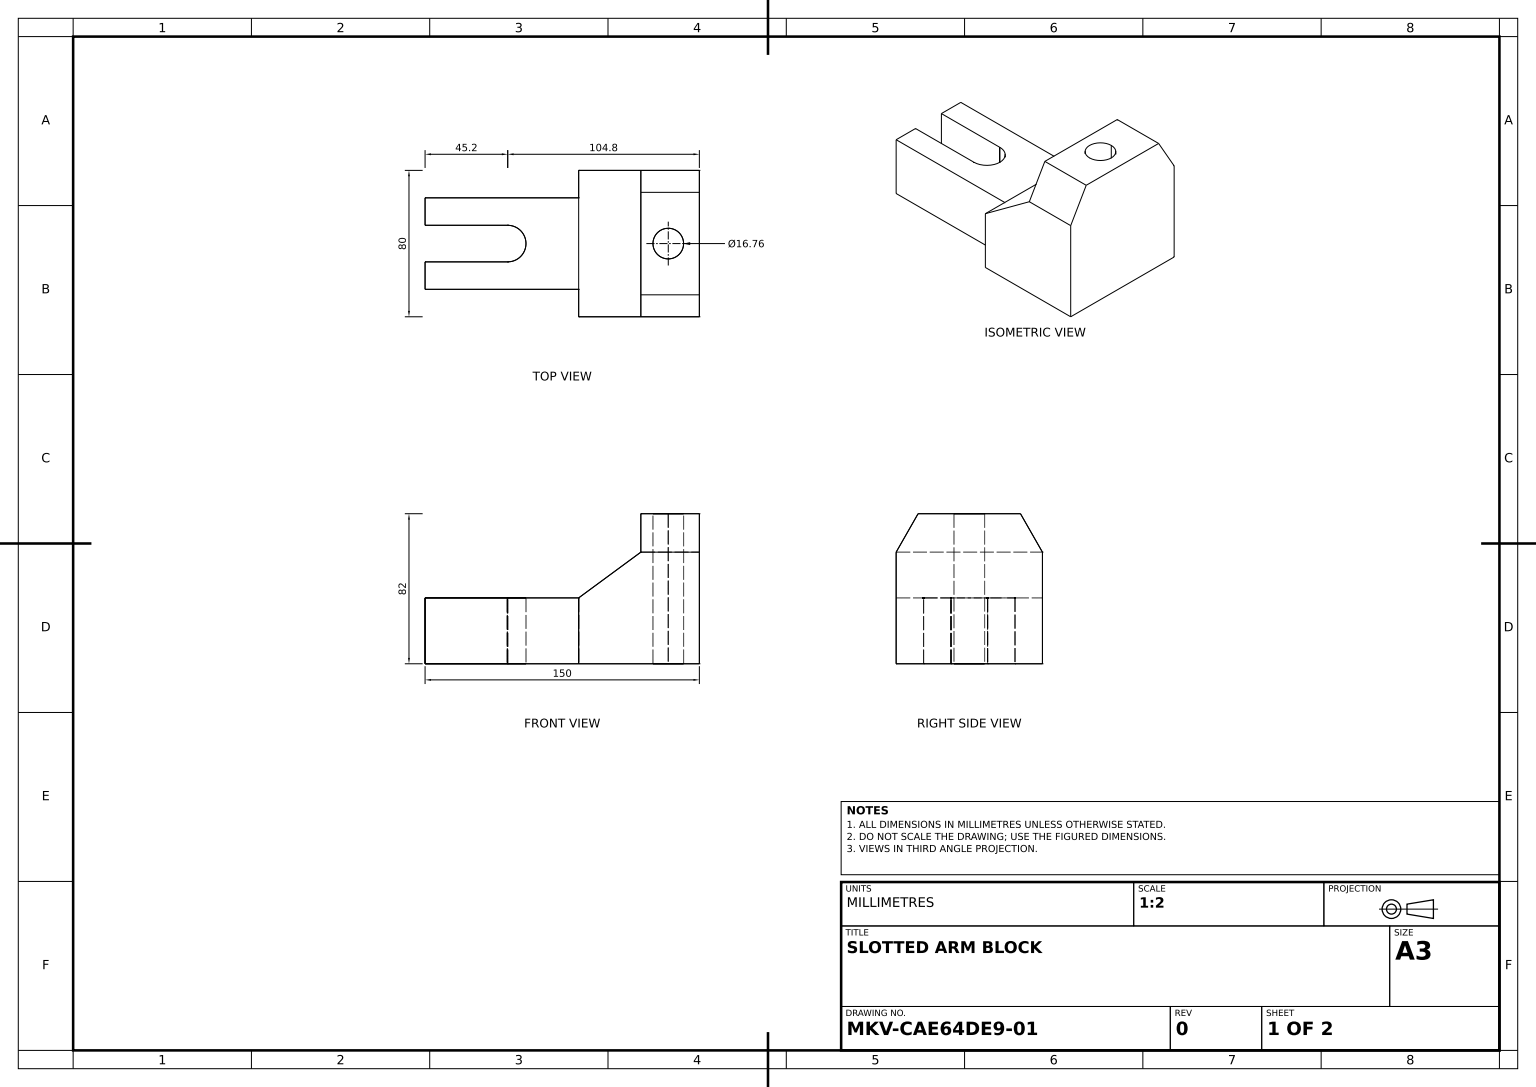
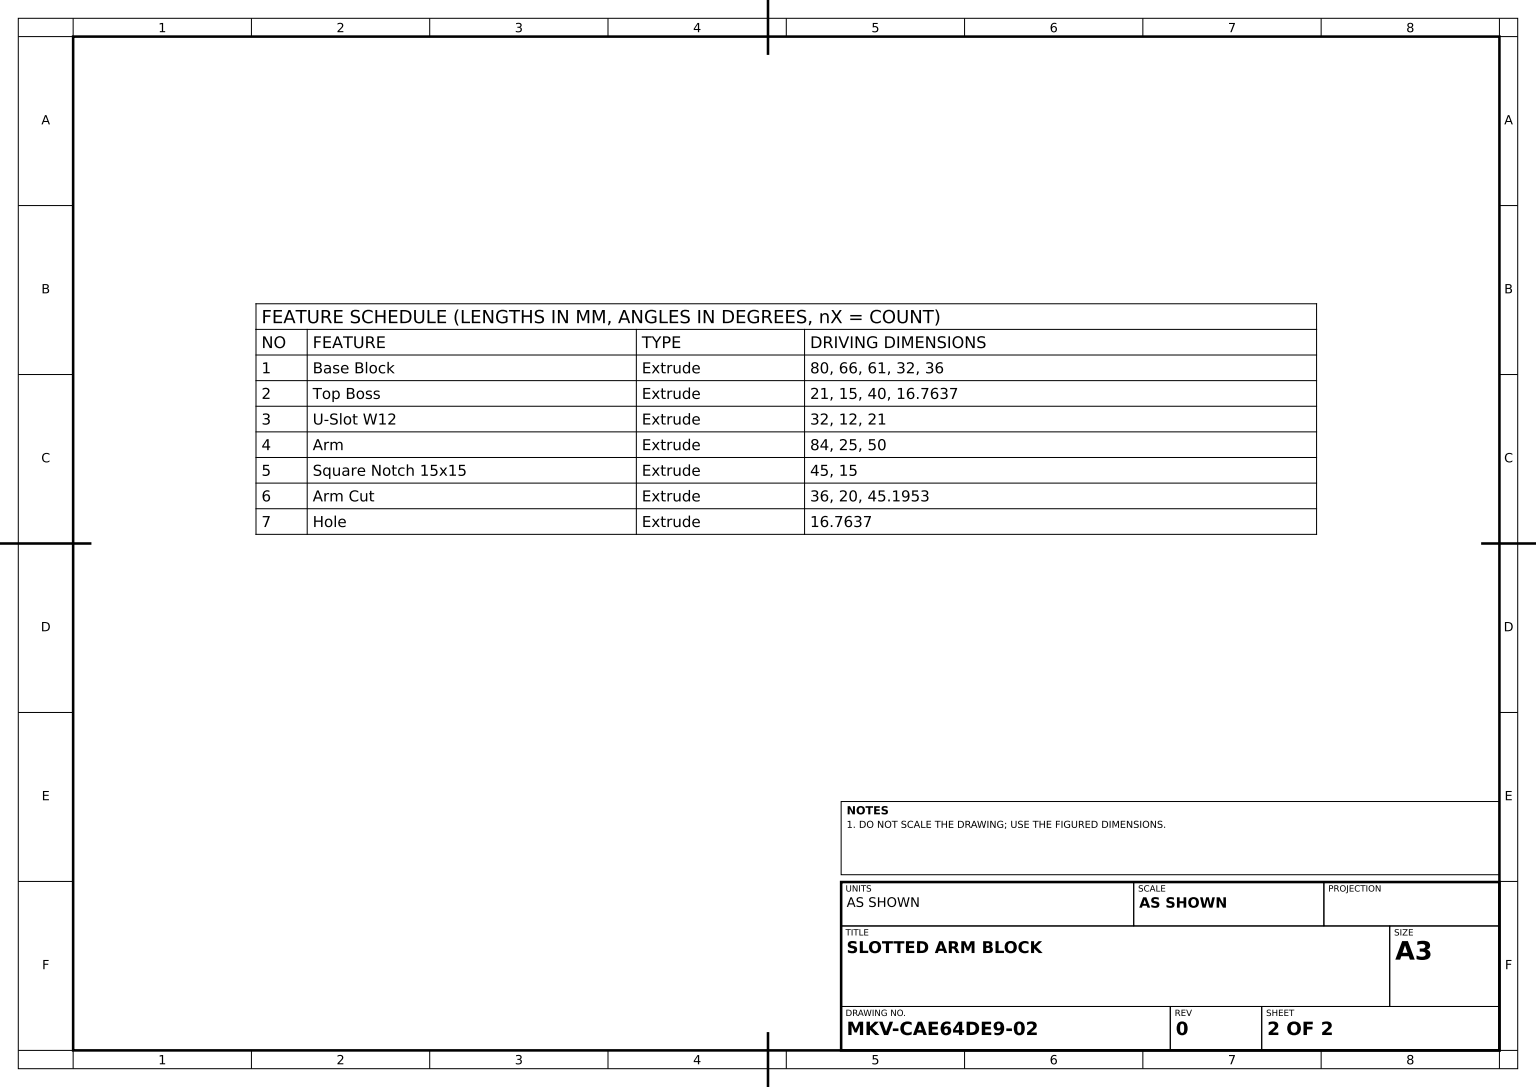
from build123d import *

# Parameters (mm, degrees)
BASE_BLOCK_DEPTH         = 40
TOP_BOSS_PROFILE_W       = 32
TOP_BOSS_PROFILE_H       = 80
TOP_BOSS_PROFILE_R       = 8.381868302
TOP_BOSS_DEPTH           = 21
U_SLOT_W12_DEPTH         = 32
ARM_PROFILE_W            = 50
ARM_PROFILE_H            = 36
ARM_DEPTH                = 84
SQUARE_NOTCH_PROFILE_W   = 20
SQUARE_NOTCH_PROFILE_H   = 36
SQUARE_NOTCH_15X15_DEPTH = 45
ARM_CUT_PROFILE_R        = 10
ARM_CUT_DEPTH            = 36
HOLE_SKETCH_R            = 8.381868302
HOLE_DEPTH               = 125.016127983


with BuildPart() as part:
    # Base Block Profile → Base Block (new, symmetric)
    with BuildSketch(Plane.XY):
        Polygon((0, 0), (0, 36), (34, 61), (66, 61), (66, 0), align=None)
    extrude(amount=BASE_BLOCK_DEPTH, both=True)

    # Top Boss Profile → Top Boss (add)
    with BuildSketch(Plane(origin=(0, 61, 0), x_dir=(1, 0, 0), z_dir=(0, 1, 0))):
        with Locations((50, 0)):
            Rectangle(TOP_BOSS_PROFILE_W, TOP_BOSS_PROFILE_H)
        with Locations(Location((49, 0, 0), (0, 0, 90))):
            Circle(TOP_BOSS_PROFILE_R, mode=Mode.SUBTRACT)
    extrude(amount=TOP_BOSS_DEPTH)

    # U-Slot Profile → U-Slot W12 (cut)
    with BuildSketch(Plane(origin=(66, 0, 0), x_dir=(0, 0, -1), z_dir=(1, 0, 0))):
        Polygon((-40, 82), (-28, 82), (-40, 61), align=None)
        Polygon((40, 61), (28, 82), (40, 82), align=None)
    extrude(amount=-U_SLOT_W12_DEPTH, mode=Mode.SUBTRACT)

    # Arm Profile → Arm (add)
    with BuildSketch(Plane.ZY):
        with Locations((0, 18)):
            Rectangle(ARM_PROFILE_W, ARM_PROFILE_H)
    extrude(amount=ARM_DEPTH)

    # Square Notch Profile → Square Notch 15x15 (cut)
    with BuildSketch(Plane.ZY.offset(84)):
        with Locations((0, 18)):
            Rectangle(SQUARE_NOTCH_PROFILE_W, SQUARE_NOTCH_PROFILE_H)
    extrude(amount=-SQUARE_NOTCH_15X15_DEPTH, mode=Mode.SUBTRACT)

    # Arm Cut Profile → Arm Cut (cut)
    with BuildSketch(Plane(origin=(0, 36, 0), x_dir=(1, 0, 0), z_dir=(0, 1, 0))):
        with Locations((-38.804725968, 0)):
            Circle(ARM_CUT_PROFILE_R)
    extrude(amount=-ARM_CUT_DEPTH, mode=Mode.SUBTRACT)

    # Hole Sketch → Hole (cut, through all)
    with BuildSketch(Plane(origin=(0, 82, 0), x_dir=(1, 0, 0), z_dir=(0, 1, 0))):
        with Locations(Location((49, 0, 0), (0, 0, 90))):
            Circle(HOLE_SKETCH_R)
    extrude(amount=-HOLE_DEPTH, mode=Mode.SUBTRACT)


solid = part.part
